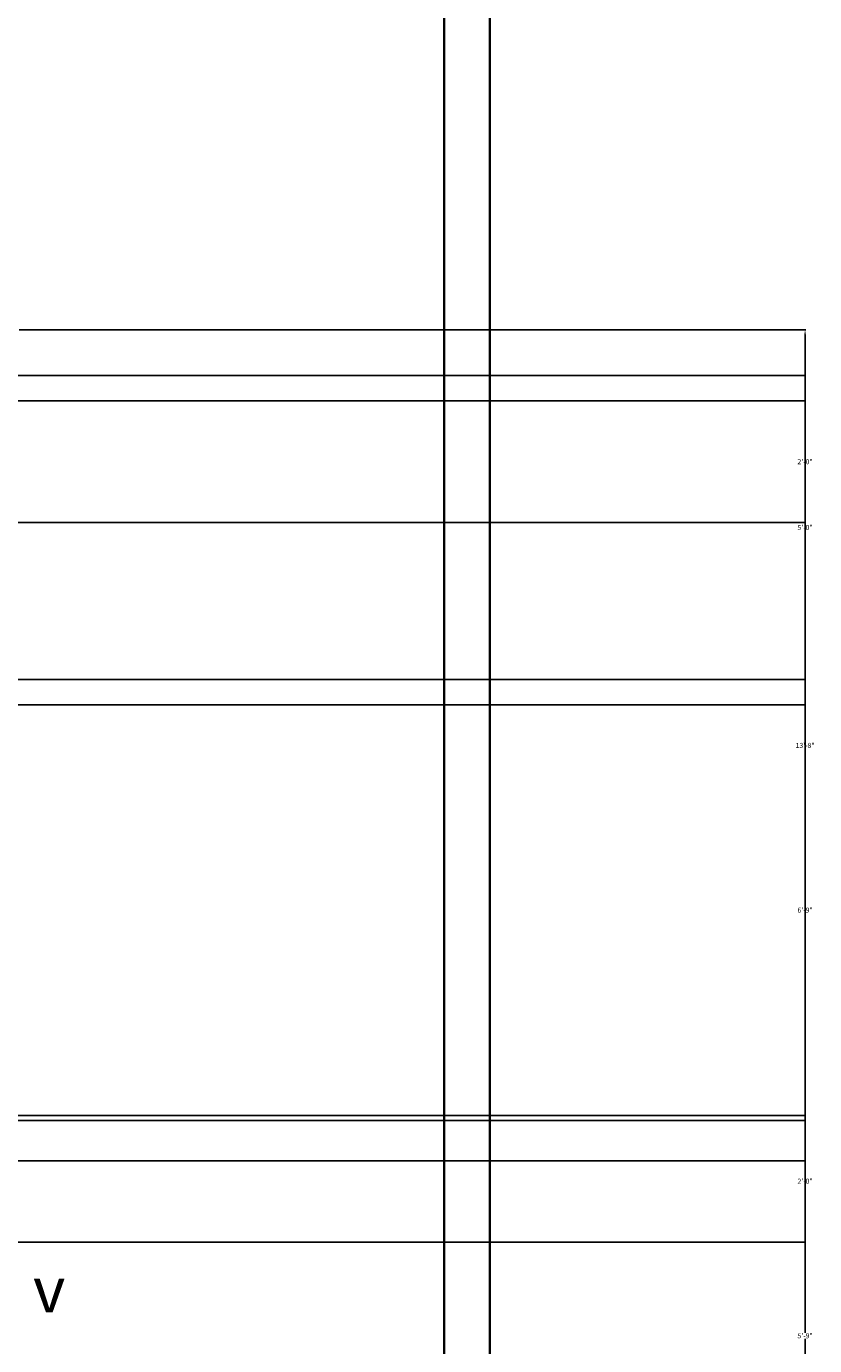
# Model space of a CAD drawing. Units: inches. Extents: x -364 to 705, y -52 to 1250.
# Tile 33 of 34: x 549 to 705, y 786 to 1046. Entities that reach past the tile are written whole.
import ezdxf

# ---------------------------------------------------------------- set-up
doc = ezdxf.new("R2010")
doc.units = ezdxf.units.IN
doc.header["$MEASUREMENT"] = 0
for name, color, linetype, lineweight in [('A-ANNO-DIMS', 4, 'Continuous', 18), ('A-ANNO-IDEN', 1, 'Continuous', 18), ('C-WALL', 41, 'Continuous', 35)]:
    doc.layers.add(name, color=color, linetype=linetype, lineweight=lineweight)
doc.styles.get("Standard").update_dxf_attribs({"font": 'arial.ttf'})
doc.dimstyles.get("Standard").update_dxf_attribs({"dimtxt": 1, "dimasz": 1, "dimexe": 0.18, "dimexo": 0.0625, "dimgap": 0.09, "dimtad": 0, "dimtih": 1, "dimtoh": 1, "dimdec": 0, "dimzin": 0, "dimdsep": 46, "dimlunit": 3, "dimtxsty": 'Standard', "dimcen": 0.09, "dimadec": 0, "dimazin": 0, "dimtfac": 1, "dimtdec": 0, "dimtofl": 0, "dimtmove": 0, "dimatfit": 3, "dimfxl": 1, "dimtolj": 1, "dimtzin": 0, "dimarcsym": 0})

# ---------------------------------------------------------------- blocks, each defined once
blk = doc.blocks.new('*D83')
at = {"layer": 'A-ANNO-DIMS', "color": 0, "lineweight": -2, "transparency": 16777216}
for p, q in [((538.64, 822.11), (703.01, 822.11)), ((702.83, 821.11), (702.83, 788.22)), ((702.83, 754.11), (702.83, 787.01)), ((538.64, 753.11), (703.01, 753.11))]:
    blk.add_line(p, q, dxfattribs=at)
at = {"layer": 'A-ANNO-DIMS', "color": 0, "transparency": 16777216}
for points in [[(702.66, 821.11), (703, 821.11), (702.83, 822.11)], [(702.66, 754.11), (703, 754.11), (702.83, 753.11)]]:
    blk.add_solid(points, dxfattribs=at)
at = {"layer": 'Defpoints', "color": 0, "transparency": 16777216}
for p in [(538.58, 822.11), (702.83, 822.11), (538.58, 753.11)]:
    blk.add_point(p, dxfattribs=at)
at = {"layer": 'A-ANNO-DIMS', "color": 0, "transparency": 16777216, "insert": (702.83, 787.61), "char_height": 1, "attachment_point": 5}
blk.add_mtext('\\A1;5\'-9"', dxfattribs=at)
blk = doc.blocks.new('*D84')
at = {"layer": 'A-ANNO-DIMS', "color": 0, "lineweight": -2, "transparency": 16777216}
for p, q in [((547.64, 986.11), (703.01, 986.11)), ((702.83, 985.11), (702.83, 904.72)), ((702.83, 823.11), (702.83, 903.51)), ((538.64, 822.11), (703.01, 822.11))]:
    blk.add_line(p, q, dxfattribs=at)
at = {"layer": 'A-ANNO-DIMS', "color": 0, "transparency": 16777216}
for points in [[(702.66, 985.11), (703, 985.11), (702.83, 986.11)], [(702.66, 823.11), (703, 823.11), (702.83, 822.11)]]:
    blk.add_solid(points, dxfattribs=at)
at = {"layer": 'Defpoints', "color": 0, "transparency": 16777216}
for p in [(547.58, 986.11), (702.83, 986.11), (538.58, 822.11)]:
    blk.add_point(p, dxfattribs=at)
at = {"layer": 'A-ANNO-DIMS', "color": 0, "transparency": 16777216, "insert": (702.83, 904.11), "char_height": 1, "attachment_point": 5}
blk.add_mtext('\\A1;13\'-8"', dxfattribs=at)
blk = doc.blocks.new('*D95')
at = {"layer": 'A-ANNO-DIMS', "color": 0, "lineweight": -2, "transparency": 16777216}
for p, q in [((103.64, 972.11), (703.01, 972.11)), ((702.83, 971.11), (702.83, 960.72)), ((702.83, 949.11), (702.83, 959.51)), ((103.64, 948.11), (703.01, 948.11))]:
    blk.add_line(p, q, dxfattribs=at)
at = {"layer": 'A-ANNO-DIMS', "color": 0, "transparency": 16777216}
for points in [[(702.66, 971.11), (703, 971.11), (702.83, 972.11)], [(702.66, 949.11), (703, 949.11), (702.83, 948.11)]]:
    blk.add_solid(points, dxfattribs=at)
at = {"layer": 'Defpoints', "color": 0, "transparency": 16777216}
for p in [(103.58, 972.11), (702.83, 972.11), (103.58, 948.11)]:
    blk.add_point(p, dxfattribs=at)
at = {"layer": 'A-ANNO-DIMS', "color": 0, "transparency": 16777216, "insert": (702.83, 960.11), "char_height": 1, "attachment_point": 5}
blk.add_mtext('\\A1;2\'-0"', dxfattribs=at)
blk = doc.blocks.new('*D96')
at = {"layer": 'A-ANNO-DIMS', "color": 0, "lineweight": -2, "transparency": 16777216}
for p, q in [((358.64, 977.11), (703.01, 977.11)), ((702.83, 976.11), (702.83, 947.72)), ((702.83, 918.11), (702.83, 946.51)), ((358.64, 917.11), (703.01, 917.11))]:
    blk.add_line(p, q, dxfattribs=at)
at = {"layer": 'A-ANNO-DIMS', "color": 0, "transparency": 16777216}
for points in [[(702.66, 976.11), (703, 976.11), (702.83, 977.11)], [(702.66, 918.11), (703, 918.11), (702.83, 917.11)]]:
    blk.add_solid(points, dxfattribs=at)
at = {"layer": 'Defpoints', "color": 0, "transparency": 16777216}
for p in [(358.58, 977.11), (358.58, 917.11), (702.83, 917.11)]:
    blk.add_point(p, dxfattribs=at)
at = {"layer": 'A-ANNO-DIMS', "color": 0, "transparency": 16777216, "insert": (702.83, 947.11), "char_height": 1, "attachment_point": 5}
blk.add_mtext('\\A1;5\'-0"', dxfattribs=at)
blk = doc.blocks.new('*D97')
at = {"layer": 'A-ANNO-DIMS', "color": 0, "lineweight": -2, "transparency": 16777216}
for p, q in [((358.64, 912.11), (703.01, 912.11)), ((702.83, 911.11), (702.83, 872.22)), ((702.83, 832.11), (702.83, 871.01)), ((358.64, 831.11), (703.01, 831.11))]:
    blk.add_line(p, q, dxfattribs=at)
at = {"layer": 'A-ANNO-DIMS', "color": 0, "transparency": 16777216}
for points in [[(702.66, 911.11), (703, 911.11), (702.83, 912.11)], [(702.66, 832.11), (703, 832.11), (702.83, 831.11)]]:
    blk.add_solid(points, dxfattribs=at)
at = {"layer": 'Defpoints', "color": 0, "transparency": 16777216}
for p in [(358.58, 912.11), (358.58, 831.11), (702.83, 831.11)]:
    blk.add_point(p, dxfattribs=at)
at = {"layer": 'A-ANNO-DIMS', "color": 0, "transparency": 16777216, "insert": (702.83, 871.61), "char_height": 1, "attachment_point": 5}
blk.add_mtext('\\A1;6\'-9"', dxfattribs=at)
blk = doc.blocks.new('*D105')
at = {"layer": 'A-ANNO-DIMS', "color": 0, "lineweight": -2, "transparency": 16777216}
for p, q in [((148.64, 830.11), (703.01, 830.11)), ((702.83, 829.11), (702.83, 818.72)), ((702.83, 807.11), (702.83, 817.51)), ((148.64, 806.11), (703.01, 806.11))]:
    blk.add_line(p, q, dxfattribs=at)
at = {"layer": 'A-ANNO-DIMS', "color": 0, "transparency": 16777216}
for points in [[(702.66, 829.11), (703, 829.11), (702.83, 830.11)], [(702.66, 807.11), (703, 807.11), (702.83, 806.11)]]:
    blk.add_solid(points, dxfattribs=at)
at = {"layer": 'Defpoints', "color": 0, "transparency": 16777216}
for p in [(148.58, 830.11), (148.58, 806.11), (702.83, 806.11)]:
    blk.add_point(p, dxfattribs=at)
at = {"layer": 'A-ANNO-DIMS', "color": 0, "transparency": 16777216, "insert": (702.83, 818.11), "char_height": 1, "attachment_point": 5}
blk.add_mtext('\\A1;2\'-0"', dxfattribs=at)

msp = doc.modelspace()

# ---------------------------------------------------------------- linework, layer by layer
at = {"layer": 'C-WALL'}
for p, q in [((640.58, 11.11), (640.58, 1079.11)), ((631.58, 11.11), (631.58, 1070.11))]:
    msp.add_line(p, q, dxfattribs=at)

# ---------------------------------------------------------------- texts
at = {"layer": 'A-ANNO-IDEN', "insert": (550.35, 801.23), "char_height": 9, "attachment_point": 1}
msp.add_mtext_dynamic_manual_height_columns('v', width=10.6887, gutter_width=1, heights=[0], dxfattribs=at)

# ---------------------------------------------------------------- dimensions: what is measured, and where the dimension line sits
at = {"layer": 'A-ANNO-DIMS'}
for base, p1, p2, picture, middle in [((702.83, 986.11), (538.58, 822.11), (547.58, 986.11), '*D84', (702.83, 904.11)), ((702.83, 917.11), (358.58, 977.11), (358.58, 917.11), '*D96', (702.83, 947.11)), ((702.83, 972.11), (103.58, 948.11), (103.58, 972.11), '*D95', (702.83, 960.11)), ((702.83, 831.11), (358.58, 912.11), (358.58, 831.11), '*D97', (702.83, 871.61)), ((702.83, 806.11), (148.58, 830.11), (148.58, 806.11), '*D105', (702.83, 818.11)), ((702.83, 822.11), (538.58, 753.11), (538.58, 822.11), '*D83', (702.83, 787.61))]:
    dim = msp.add_linear_dim(base=base, p1=p1, p2=p2, angle=90, dimstyle='Standard', override={"dimdec": 1, "dimlfac": 1, "dimrnd": 0, "dimzin": 1, "dimdsep": 46, "dimlunit": 4, "dimfrac": 2}, dxfattribs=at)
    dim.commit()
    dim.dimension.update_dxf_attribs({"geometry": picture, "text_midpoint": middle})

doc.saveas('drawing.dxf')
